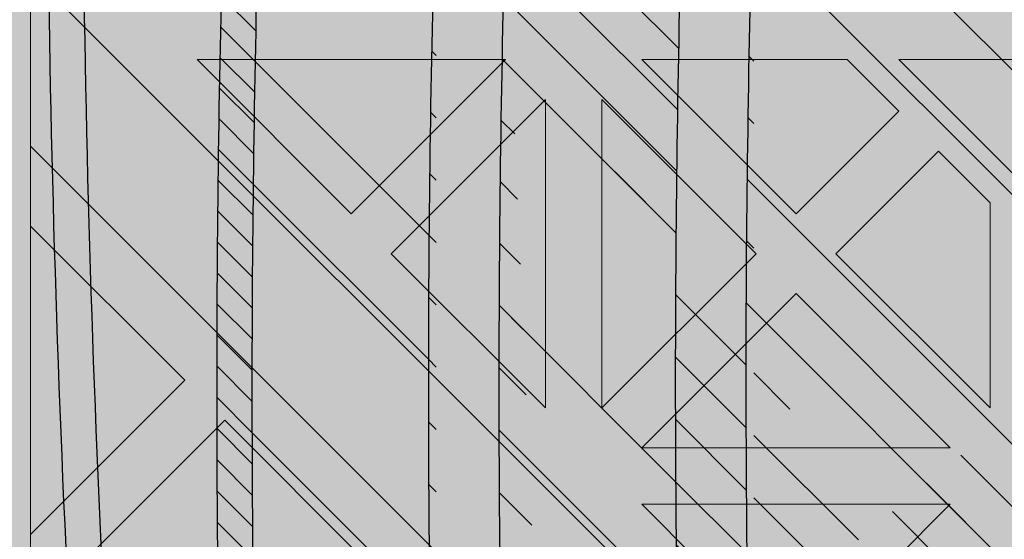
# Model space of a CAD drawing. Units: inches. Extents: x 844 to 2234, y 346 to 1084.
# Tile 28 of 93: x 1252.862 to 1257.311, y 693.415 to 695.763. Entities that reach past the tile are written whole.
import ezdxf

# ---------------------------------------------------------------- set-up
doc = ezdxf.new("R2010")
doc.units = ezdxf.units.IN
doc.header["$MEASUREMENT"] = 0
doc.layers.add('furniture', color=8, linetype='Continuous', lineweight=18)
doc.layers.add('RA-AP-01$0$INT', color=35, linetype='Continuous', lineweight=5)
doc.layers.add('RA-AP-01$0$FURN', color=3, linetype='Continuous')
doc.layers.add('RA-AP-01$0$WOOD', color=64, linetype='Continuous')

# ---------------------------------------------------------------- blocks, each defined once
blk = doc.blocks.new('A$C18D01794')
at = {"layer": 'RA-AP-01$0$INT'}
blk.add_hatch(color=256, dxfattribs=at).paths.add_polyline_path([(4.505206456958071, -6.306712009588038), (5.305206456958072, -6.306712009588038), (5.305206456958072, -7.106712009588038), (5.255206456951893, -7.10671200958804), (5.25520645694868, -6.356712009605972), (4.555206456959269, -6.356712009587461), (4.555206456956052, -7.106712009588038), (4.505206456958073, -7.106712009588038)])
h = blk.add_hatch(color=256, dxfattribs=at)
h.paths.add_polyline_path([(4.585917135068449, -6.356712009588271), (4.555206456959269, -6.35671200958746), (4.555206456959137, -6.387422687716308), (4.874495778835233, -6.706712009592356), (4.90520645695423, -6.676001331474049)])
h.paths.add_polyline_path([(5.255206456948813, -6.387422687716306), (5.255206456948682, -6.356712009605972), (5.224495778822613, -6.356712009605161), (4.905206456953498, -6.676001331474273), (4.935917135072151, -6.706712009592924)])
h.paths.add_polyline_path([(4.935917135072559, -6.706712009592068), (4.905206456953564, -6.737422687710376), (5.255206456951813, -7.087422687708613), (5.255206456951549, -7.026001331471008)])
h.paths.add_polyline_path([(4.555206456956399, -7.026001331471013), (4.555206456956134, -7.087422687708616), (4.905206456953821, -6.737422687710943), (4.874495778835166, -6.70671200959229)])
h = blk.add_hatch(color=256, dxfattribs=at)
h.paths.add_polyline_path([(4.585917135068448, -6.356712009588273), (4.614201406330596, -6.356712009589021), (4.668846067270487, -6.411356670531338), (4.723490728212344, -6.356712009591912), (4.771774999457151, -6.35671200959319), (4.826419660396886, -6.411356670535356), (4.862780050090322, -6.374996280843536), (4.844495778842715, -6.356712009595112), (4.862780050090411, -6.356712009595595), (4.905206456960182, -6.399138416468211), (4.947632863832445, -6.356712009597838), (4.965917135079675, -6.356712009598322), (4.947632863831759, -6.374996280845421), (4.983993253523576, -6.411356670538857), (5.038637914464627, -6.356712009600247), (5.08692218571208, -6.356712009601523), (5.141566846649976, -6.411356670541852), (5.196211507589851, -6.356712009604411), (5.224495778822615, -6.356712009605161), (4.905206456953975, -6.676001331473793)])
h.paths.add_polyline_path([(4.895206456956031, -6.637717060225675), (4.895206456958921, -6.528427738347902), (4.840561796018589, -6.583072399285802)], flags=16)
h.paths.add_polyline_path([(4.915206456955638, -6.637717060226121), (4.969851117895509, -6.583072399288678), (4.915206456957609, -6.528427738348344)], flags=16)
h.paths.add_polyline_path([(4.826419660395175, -6.568930263661755), (4.881064321335613, -6.514285602723745), (4.771774999456703, -6.514285602720857)], flags=16)
h.paths.add_polyline_path([(4.983993253519558, -6.568930263665262), (5.038637914460456, -6.514285602726792), (4.929348592581548, -6.514285602724816)], flags=16)
h.paths.add_polyline_path([(4.881064321336025, -6.494285602723742), (4.826419660397532, -6.439640941782821), (4.771774999457062, -6.494285602720859)], flags=16)
h.paths.add_polyline_path([(4.929348592582019, -6.494285602724817), (5.038637914460982, -6.494285602726792), (4.983993253522945, -6.439640941786327)], flags=16)
h.paths.add_polyline_path([(4.895206456960191, -6.480143467100443), (4.895206456962115, -6.407422687715913), (4.876922185715016, -6.389138416467584), (4.840561796021581, -6.425498806159401)], flags=16)
h.paths.add_polyline_path([(4.915206456958487, -6.480143467100889), (4.969851117899527, -6.425498806162279), (4.933490728206909, -6.389138416468043), (4.9152064569598, -6.40742268771434)], flags=16)
h.paths.add_polyline_path([(4.757632863832376, -6.480143467096812), (4.812277524772842, -6.425498806158772), (4.757632863834348, -6.370854145217844)], flags=16)
h.paths.add_polyline_path([(4.737632863832376, -6.480143467096286), (4.737632863834348, -6.370854145217375), (4.682988202893906, -6.425498806155385)], flags=16)
h.paths.add_polyline_path([(5.05278005008503, -6.480143467103376), (5.052780050087917, -6.370854145224413), (4.998135389146995, -6.425498806162908)], flags=16)
h.paths.add_polyline_path([(5.072780050085024, -6.480143467103744), (5.127424711025931, -6.42549880616527), (5.072780050087916, -6.370854145224832)], flags=16)
h.paths.add_polyline_path([(4.935917135072783, -6.706712009592292), (5.255206456948811, -6.387422687716309), (5.255206456948932, -6.415706958964177), (5.200561796010279, -6.470351619902839), (5.255206456949403, -6.524996280841948), (5.25520645694961, -6.5732805520894), (5.200561796009787, -6.627925213029239), (5.236922185702417, -6.664285602721864), (5.255206456949919, -6.646001331474357), (5.255206456949998, -6.664285602721898), (5.212780050078687, -6.706712009592262), (5.25520645695036, -6.749138416463932), (5.255206456950438, -6.767422687711313), (5.236922185702424, -6.749138416463297), (5.200561796009796, -6.785498806155928), (5.255206456950753, -6.840143467096874), (5.25520645695096, -6.888427738341682), (5.200561796010322, -6.943072399282328), (5.255206456951428, -6.997717060223427), (5.255206456951547, -7.026001331471006)])
h.paths.add_polyline_path([(5.042988202883395, -6.785498806155427), (5.097632863823085, -6.840143467095101), (5.097632863822622, -6.730854145216193)], flags=16)
h.paths.add_polyline_path([(5.028846067259663, -6.771356670531693), (5.083490728198774, -6.716712009592573), (4.974201406321001, -6.716712009593042)], flags=16)
h.paths.add_polyline_path([(5.117632863823087, -6.840143467095186), (5.172277524762331, -6.785498806155926), (5.11763286382262, -6.730854145216225)], flags=16)
h.paths.add_polyline_path([(5.08349072819877, -6.696712009593886), (5.028846067259652, -6.642067348654775), (4.974201406320998, -6.696712009593438)], flags=16)
h.paths.add_polyline_path([(5.131774999446817, -6.854285602718917), (5.186419660386065, -6.799640941779662), (5.241064321325782, -6.854285602719365)], flags=17)
h.paths.add_polyline_path([(5.131774999446228, -6.716712009592374), (5.186419660386065, -6.771356670532194), (5.222780050079488, -6.734996280838764), (5.204495778832781, -6.716712009592063)], flags=16)
h.paths.add_polyline_path([(5.097632863822613, -6.682569873970264), (5.097632863823061, -6.573280552091354), (5.042988202883383, -6.627925213031044)], flags=16)
h.paths.add_polyline_path([(5.131774999446899, -6.874285602718915), (5.241064321325809, -6.874285602719364), (5.186419660386591, -6.928930263658598)], flags=17)
h.paths.add_polyline_path([(5.131774999446226, -6.696712009594078), (5.204495778830767, -6.696712009594374), (5.22278005007868, -6.67842773834687), (5.186419660386049, -6.642067348654249)], flags=16)
h.paths.add_polyline_path([(5.11763286382262, -6.682569873970225), (5.17227752476232, -6.627925213030515), (5.117632863823064, -6.573280552091267)], flags=16)
h.paths.add_polyline_path([(5.186419660386069, -6.613783077405491), (5.241064321325754, -6.559138416465795), (5.131774999446791, -6.559138416466263)], flags=16)
h.paths.add_polyline_path([(5.131774999446872, -6.539138416466263), (5.24106432132578, -6.539138416465794), (5.186419660386554, -6.484493755526573)], flags=16)
h.paths.add_polyline_path([(5.255206456951811, -7.08742268770861), (5.255206456951895, -7.106712009588038), (4.555206456956052, -7.106712009588038), (4.555206456956136, -7.087422687708617), (4.905206456953973, -6.737422687710788)])
h.paths.add_polyline_path([(4.983993253513404, -6.8444937555241), (4.92934859257295, -6.899138416462108), (5.03863791445186, -6.899138416465014)], flags=16)
h.paths.add_polyline_path([(4.969851117889988, -6.83035161990006), (4.915206456952556, -6.775706958960171), (4.915206456949648, -6.884996280837944)], flags=16)
h.paths.add_polyline_path([(4.929348592572535, -6.919138416462105), (4.983993253511019, -6.973783077403037), (5.038637914451496, -6.919138416465012)], flags=16)
h.paths.add_polyline_path([(5.052780050074912, -6.93328055208906), (4.998135389134438, -6.987925213027088), (5.052780050072919, -7.042569873968025)], flags=16)
h.paths.add_polyline_path([(5.07278005007491, -6.933280552089588), (5.072780050072918, -7.042569873968497), (5.127424711013374, -6.987925213030498)], flags=16)
h.paths.add_polyline_path([(4.89520645695295, -6.775706958959721), (4.840561796013067, -6.830351619897157), (4.895206456950961, -6.884996280837494)], flags=16)
h.paths.add_polyline_path([(4.915206456948365, -6.933280552085403), (4.915206456946434, -7.006001331471951), (4.933490728192729, -7.024285602719066), (4.969851117886972, -6.987925213026453)], flags=16)
h.paths.add_polyline_path([(4.881064321327021, -6.899138416461022), (4.82641966038902, -6.84449375552057), (4.771774999448108, -6.899138416459029)], flags=16)
h.paths.add_polyline_path([(4.895206456950073, -6.933280552084951), (4.840561796009022, -6.987925213023558), (4.876922185700835, -7.024285602716997), (4.895206456948749, -7.006001331469487)], flags=16)
h.paths.add_polyline_path([(4.983993253510392, -7.0020673486505), (4.947632863816944, -7.038427738342319), (4.965917135064043, -7.05671200959023), (5.038637914448995, -7.056712009591555)], flags=16)
h.paths.add_polyline_path([(4.881064321326543, -6.91913841646102), (4.771774999447578, -6.919138416459031), (4.826419660385607, -6.973783077399508)], flags=16)
h.paths.add_polyline_path([(4.905206456946447, -7.014285602717636), (4.862780050074785, -7.056712009588352), (4.947632863816685, -7.056712009589775)], flags=16)
h.paths.add_polyline_path([(5.14156684663679, -7.002067348654549), (5.086922185696452, -7.056712009592438), (5.196211507574223, -7.056712009594425)], flags=16)
h.paths.add_polyline_path([(4.8264196603837, -7.002067348646972), (4.771774999442643, -7.056712009585575), (4.8444957788276, -7.056712009587508), (4.862780050075511, -7.038427738340416)], flags=16)
h.paths.add_polyline_path([(4.812277524760289, -6.98792521302292), (4.757632863822258, -6.933280552082447), (4.757632863819352, -7.042569873961408)], flags=16)
h.paths.add_polyline_path([(4.73763286382226, -6.933280552082079), (4.682988202881349, -6.987925213020536), (4.737632863819352, -7.04256987396099)], flags=16)
h.paths.add_polyline_path([(4.723490728195188, -7.056712009584289), (4.668846067257299, -7.002067348643949), (4.614201406317417, -7.056712009581383)], flags=16)
h.paths.add_polyline_path([(4.597632863829262, -6.706712009592262), (4.555206456957951, -6.664285602721896), (4.555206456958029, -6.646001331474357), (4.573490728205535, -6.664285602721864), (4.609851117898167, -6.627925213029238), (4.555206456958338, -6.573280552089402), (4.555206456958546, -6.524996280841952), (4.60985111789767, -6.470351619902839), (4.555206456959015, -6.415706958964177), (4.555206456959138, -6.387422687716309), (4.874495778835167, -6.70671200959229), (4.5552064569564, -7.026001331471015), (4.555206456956523, -6.997717060223433), (4.609851117897629, -6.94307239928233), (4.555206456956988, -6.888427738341681), (4.555206456957198, -6.840143467096881), (4.609851117898153, -6.78549880615593), (4.573490728205528, -6.749138416463297), (4.555206456957507, -6.76742268771132), (4.555206456957585, -6.749138416463933)])
h.paths.add_polyline_path([(4.712780050085332, -6.730854145216195), (4.712780050084863, -6.840143467095105), (4.767424711024555, -6.785498806155427)], flags=16)
h.paths.add_polyline_path([(4.726922185709173, -6.716712009592573), (4.781566846648288, -6.771356670531693), (4.836211507586949, -6.716712009593043)], flags=16)
h.paths.add_polyline_path([(4.692780050085327, -6.730854145216225), (4.638135389145619, -6.785498806155928), (4.692780050084865, -6.840143467095185)], flags=16)
h.paths.add_polyline_path([(4.726922185709182, -6.696712009593886), (4.836211507586949, -6.696712009593436), (4.7815668466483, -6.642067348654773)], flags=16)
h.paths.add_polyline_path([(4.678637914461726, -6.71671200959237), (4.605917135075169, -6.716712009592063), (4.587632863828464, -6.734996280838766), (4.623993253521887, -6.771356670532195)], flags=16)
h.paths.add_polyline_path([(4.712780050085336, -6.68256987397026), (4.767424711024568, -6.627925213031042), (4.71278005008489, -6.573280552091352)], flags=16)
h.paths.add_polyline_path([(4.678637914461726, -6.696712009594076), (4.623993253521899, -6.642067348654247), (4.587632863829271, -6.67842773834687), (4.605917135077185, -6.696712009594376)], flags=16)
h.paths.add_polyline_path([(4.692780050085336, -6.682569873970228), (4.692780050084889, -6.573280552091267), (4.638135389145632, -6.627925213030515)], flags=16)
h.paths.add_polyline_path([(4.623993253521885, -6.799640941779662), (4.678637914461131, -6.854285602718915), (4.56934859258217, -6.854285602719365)], flags=17)
h.paths.add_polyline_path([(4.623993253521901, -6.613783077405509), (4.678637914461158, -6.559138416466263), (4.569348592582195, -6.559138416465795)], flags=16)
h.paths.add_polyline_path([(4.678637914461051, -6.874285602718915), (4.623993253521361, -6.928930263658598), (4.569348592582143, -6.874285602719364)], flags=17)
h.paths.add_polyline_path([(4.678637914461076, -6.539138416466263), (4.623993253521399, -6.484493755526573), (4.569348592582167, -6.539138416465796)], flags=16)
h = blk.add_hatch(color=256, dxfattribs=at)
h.paths.add_polyline_path([(5.028846067259997, -6.642067348655121), (4.974201406321342, -6.696712009593783), (5.083490728199115, -6.69671200959423)])
h.paths.add_polyline_path([(4.974201406321344, -6.716712009593388), (5.028846067260004, -6.771356670532039), (5.083490728199117, -6.716712009592919)])
h.paths.add_polyline_path([(5.042988202883738, -6.785498806155768), (5.097632863823428, -6.840143467095449), (5.097632863822963, -6.73085414521654)])
h.paths.add_polyline_path([(5.117632863822961, -6.730854145216568), (5.117632863823428, -6.840143467095531), (5.172277524762674, -6.785498806156272)])
h.paths.add_polyline_path([(5.131774999446572, -6.716712009592718), (5.186419660386406, -6.77135667053254), (5.222780050079831, -6.734996280839116), (5.204495778833122, -6.716712009592409)])
h.paths.add_polyline_path([(5.236922185702764, -6.749138416463644), (5.200561796010139, -6.785498806156274), (5.255206456949971, -6.840143467096101), (5.255206456950271, -6.76742268771115)])
h.paths.add_polyline_path([(5.186419660386412, -6.799640941780006), (5.131774999447164, -6.854285602719262), (5.241064321326123, -6.854285602719711)])
h.paths.add_polyline_path([(5.131774999447238, -6.874285602719261), (5.186419660386934, -6.928930263658944), (5.241064321326153, -6.874285602719709)])
h.paths.add_polyline_path([(5.200561796010663, -6.943072399282675), (5.255206456949324, -6.997717060221329), (5.255206456949777, -6.888427738343558)])
h.paths.add_polyline_path([(5.21278005007903, -6.706712009592607), (5.255206456950223, -6.749138416463798), (5.255206456950696, -6.664285602721891)])
h.paths.add_polyline_path([(5.13177499944657, -6.696712009594424), (5.204495778831106, -6.696712009594723), (5.222780050079024, -6.678427738347219), (5.186419660386397, -6.642067348654592)])
h.paths.add_polyline_path([(5.117632863823405, -6.573280552091611), (5.117632863822955, -6.682569873970578), (5.172277524762665, -6.627925213030859)])
h.paths.add_polyline_path([(5.042988202883727, -6.627925213031387), (5.097632863822957, -6.682569873970603), (5.097632863823407, -6.573280552091697)])
h.paths.add_polyline_path([(5.131774999447135, -6.559138416466609), (5.186419660386394, -6.613783077405857), (5.241064321326097, -6.559138416466144)])
h.paths.add_polyline_path([(5.200561796010128, -6.627925213029584), (5.236922185702758, -6.664285602722211), (5.255206456950264, -6.646001331474705), (5.255206456949948, -6.573280552089752)])
h.paths.add_polyline_path([(5.186419660386895, -6.484493755526919), (5.131774999447213, -6.539138416466609), (5.241064321326127, -6.539138416466142)])
h.paths.add_polyline_path([(5.200561796010624, -6.470351619903183), (5.255206456949745, -6.524996280842298), (5.255206456949276, -6.415706958964523)])
h = blk.add_hatch(color=256, dxfattribs=at)
h.paths.add_polyline_path([(4.895206456952951, -6.77570695895972), (4.840561796013068, -6.830351619897156), (4.895206456950958, -6.884996280837495)])
h.paths.add_polyline_path([(4.915206456949649, -6.884996280837942), (4.969851117889987, -6.830351619900054), (4.915206456952556, -6.775706958960171)])
h.paths.add_polyline_path([(5.038637914451862, -6.899138416465013), (4.983993253513403, -6.8444937555241), (4.929348592572953, -6.899138416462106)])
h.paths.add_polyline_path([(4.929348592572535, -6.919138416462105), (4.983993253511018, -6.973783077403037), (5.038637914451497, -6.919138416465012)])
h.paths.add_polyline_path([(4.915206456948366, -6.933280552085397), (4.915206456946433, -7.006001331471951), (4.93349072819273, -7.024285602719068), (4.969851117886972, -6.987925213026454)])
h.paths.add_polyline_path([(5.038637914448995, -7.056712009591553), (4.983993253510389, -7.002067348650502), (4.947632863816946, -7.038427738342318), (4.965917135064043, -7.05671200959023)])
h.paths.add_polyline_path([(5.05278005007292, -7.042569873968023), (5.05278005007491, -6.933280552089059), (4.998135389134438, -6.987925213027088)])
h.paths.add_polyline_path([(5.07278005007292, -7.042569873968496), (5.127424711013374, -6.987925213030498), (5.072780050074909, -6.933280552089588)])
h.paths.add_polyline_path([(5.141566846636789, -7.002067348654547), (5.086922185696449, -7.056712009592438), (5.196211507574223, -7.056712009594425)])
h.paths.add_polyline_path([(4.947632863816688, -7.056712009589774), (4.905206456946449, -7.014285602717634), (4.862780050074784, -7.056712009588353)])
h.paths.add_polyline_path([(4.840561796009025, -6.987925213023556), (4.876922185700834, -7.024285602716997), (4.895206456948747, -7.006001331469488), (4.895206456950075, -6.933280552084953)])
h.paths.add_polyline_path([(4.88106432132654, -6.919138416461021), (4.771774999447577, -6.919138416459031), (4.826419660385606, -6.973783077399508)])
h.paths.add_polyline_path([(4.881064321327019, -6.899138416461022), (4.826419660389019, -6.844493755520571), (4.771774999448108, -6.89913841645903)])
h.paths.add_polyline_path([(4.757632863819352, -7.042569873961409), (4.812277524760284, -6.987925213022922), (4.757632863822259, -6.933280552082447)])
h.paths.add_polyline_path([(4.8264196603837, -7.002067348646974), (4.771774999442646, -7.056712009585575), (4.844495778827599, -7.05671200958751), (4.862780050075512, -7.038427738340417)])
h.paths.add_polyline_path([(4.737632863819352, -7.042569873960988), (4.737632863822258, -6.933280552082078), (4.682988202881349, -6.987925213020538)])
h.paths.add_polyline_path([(4.668846067257299, -7.002067348643952), (4.61420140631742, -7.056712009581384), (4.723490728195189, -7.056712009584292)])
for p, q in [((5.255206456951895, -7.106712009588038), (5.255206456948681, -6.356712009605972)), ((4.935917135072783, -6.706712009592292), (5.255206456951548, -7.026001331471007)), ((4.905206456953975, -6.737422687710788), (5.255206456951811, -7.087422687708611)), ((4.929348592572952, -6.899138416462106), (4.983993253513403, -6.844493755524101)), ((4.983993253513404, -6.844493755524103), (5.038637914451862, -6.899138416465012)), ((5.186419660386587, -6.928930263658596), (5.131774999446899, -6.874285602718915)), ((5.241064321325809, -6.874285602719364), (5.186419660386589, -6.928930263658598)), ((5.255206456949429, -6.888427738343214), (5.200561796010322, -6.943072399282328)), ((5.255206456949433, -6.888427738343212), (5.255206456948982, -6.997717060220983)), ((5.038637914451862, -6.899138416465012), (4.929348592572952, -6.899138416462106)), ((5.038637914451498, -6.919138416465012), (4.929348592572535, -6.919138416462105)), ((4.929348592572535, -6.919138416462105), (4.983993253511019, -6.973783077403037)), ((5.038637914451498, -6.919138416465012), (4.983993253511019, -6.973783077403037)), ((4.915206456946434, -7.006001331470351), (4.915206456948367, -6.933280552085399)), ((4.915206456948367, -6.933280552085399), (4.969851117886972, -6.987925213026453)), ((5.05278005007491, -6.93328055208906), (4.998135389134438, -6.987925213027088)), ((5.05278005007491, -6.93328055208906), (5.052780050072921, -7.042569873968023)), ((5.127424711013373, -6.987925213030496), (5.07278005007491, -6.933280552089588)), ((5.07278005007491, -6.933280552089588), (5.07278005007292, -7.042569873968497)), ((5.255206456948982, -6.997717060220983), (5.200561796010322, -6.943072399282328)), ((4.969851117886972, -6.987925213026452), (4.93349072819353, -7.024285602718265)), ((5.052780050072921, -7.042569873968023), (4.998135389134438, -6.987925213027088)), ((5.07278005007292, -7.042569873968497), (5.127424711013374, -6.987925213030498)), ((4.98399325351039, -7.002067348650502), (4.947632863816946, -7.038427738342317)), ((5.038637914448995, -7.056712009591555), (4.983993253510388, -7.002067348650502)), ((5.086922185696454, -7.056712009592434), (5.141566846636789, -7.002067348654547)), ((5.196211507574223, -7.056712009594425), (5.141566846636789, -7.002067348654547)), ((4.915206456946427, -7.006001331471944), (4.933490728193524, -7.02428560271986)), ((4.905206456946449, -7.014285602717635), (4.94763286381669, -7.056712009589775)), ((4.947632863816946, -7.038427738342317), (4.965917135063997, -7.056712009590183)), ((4.965917135064043, -7.056712009590231), (4.947632863816944, -7.038427738342317)), ((4.94763286381669, -7.056712009589775), (4.862780050074783, -7.056712009588354)), ((4.965917135064043, -7.05671200959023), (5.038637914448995, -7.056712009591555)), ((5.086922185696452, -7.056712009592438), (5.196211507574223, -7.056712009594425))]:
    blk.add_line(p, q, dxfattribs=at)
blk = doc.blocks.new('A$C32926AE1')
at = {"layer": 'RA-AP-01$0$FURN'}
h = blk.add_hatch(dxfattribs=at)
h.set_pattern_fill('ANSI31', color=256, scale=0.1, style=0)
h.set_pattern_definition([(45, (0, 0), (-0.0088388347648318, 0.0088388347648318), [])])
edge = h.paths.add_edge_path(flags=16)
edge.add_arc((4.904771284329206, 4.246793130718756), 0.2603971832811541, 75.22398030683196, 104.7760196931204)
edge.add_arc((4.904771284329206, 4.246793130718756), 0.2603971832811541, 75.223980306832, 104.77601969312039, ccw=False)
edge = h.paths.add_edge_path(flags=16)
edge.add_arc((4.904771284329206, 4.067062675376612), 0.2603971832811541, 255.2239803068796, 284.776019693168)
edge.add_arc((4.904771284329206, 4.067062675376612), 0.2603971832811541, 255.22398030687958, 284.77601969316805, ccw=False)
edge = h.paths.add_edge_path(flags=0)
edge.add_arc((4.904771284329206, 4.067062675376612), 0.2603971832811541, 255.2239803068796, 284.776019693168)
edge.add_arc((4.904771284329206, 4.067062675376612), 0.2603971832811541, 255.22398030687958, 284.77601969316805, ccw=False)
edge = h.paths.add_edge_path(flags=0)
edge.add_arc((4.904771284329206, 4.067062675376612), 0.2603971832811541, 255.2239803068796, 284.776019693168)
edge.add_arc((4.904771284329206, 4.067062675376612), 0.2603971832811541, 255.22398030687958, 284.77601969316805, ccw=False)
edge = h.paths.add_edge_path()
edge.add_arc((4.604388392048174, 4.588829985554312), 0.1599999999999918, 342.3781640246255, 354.4317409793762)
edge.add_arc((5.090145208887507, 4.43216705527679), 0.3503971832811637, 162.0091218307731, 180.3186872093483)
edge.add_arc((5.205154176610243, 4.588829985554953), 0.1599999999999917, 185.5682590208461, 197.6218359767349)
edge.add_arc((4.904771284329229, 4.246793130718735), 0.3503971832811761, 72.00912183053516, 107.9908781690354)
edge.add_arc((9.535952835716557, 4.28682295566602), 4.798342501046485, 178.2875002453811, 181.5576802719453)
edge.add_arc((4.719397359771122, 4.43216705527679), 0.3503971832811637, 359.6813127906516, 377.9908781692269)
edge.add_arc((9.535967292294904, 4.286822350292874), 4.778371420254705, 178.2965938931842, 181.5667745797229)
edge.add_arc((4.719397359771122, 4.43216705527679), 0.3303971832811637, 359.6813127906516, 377.9908781692269)
edge.add_arc((0.2735752763637294, 4.286822350292874), 4.7783714202547, 358.4332254202771, 361.7034061068158)
edge.add_arc((5.061434214606998, 4.732549947558029), 0.1600000000000254, 252.3781640250584, 264.4317409792362)
edge.add_arc((4.748108354051257, 4.732549947558012), 0.1600000000000541, 275.5682590208426, 287.6218359759532)
edge.add_arc((4.604388392048115, 4.588829985554317), 0.1800000000000505, 342.3567572500182, 349.3735009646207)
edge.add_arc((5.205154176610254, 4.588829985554976), 0.1800000000000069, 190.6264990356027, 197.6432427513933)
edge.add_arc((5.061434214607106, 4.732549947558013), 0.1800000000000424, 252.3567572496606, 259.3735009644582)
edge.add_arc((4.904771284329208, 4.246793130718737), 0.3303971832811676, 71.99844483668534, 108.0015551637021)
edge.add_arc((4.748108354051414, 4.732549947558045), 0.1800000000000547, 280.6264990355479, 287.6432427495938)
edge.add_arc((5.090145208887514, 4.432167055276789), 0.2803971832811691, 162.8706300666893, 180.816523289902)
edge.add_arc((4.719397359771136, 4.432167055276689), 0.2803971832811534, 359.183476710103, 377.1293699333214)
edge.add_arc((4.904771284329222, 4.246793130718737), 0.2803971832811769, 72.87063006672916, 107.1293699332334)
edge.add_arc((5.090145208887522, 4.432167055276788), 0.2603971832811776, 165.2239803068007, 180.9953123810312)
edge.add_arc((4.719397359771141, 4.432167055276699), 0.2603971832811458, 359.0046876189768, 374.7760196932087)
edge.add_arc((5.090145208887507, 4.43216705527679), 0.3303971832811637, 162.0091218307731, 180.3186872093483)
edge.add_arc((9.53595427642584, 4.285015535491528), 4.728345371032053, 178.265043920078, 181.5679956281801)
edge.add_arc((0.2735882922327999, 4.285015535491582), 4.728345371032045, 358.4320043718193, 361.7349560799204)
edge.add_arc((9.535953591267507, 4.284458026472751), 4.708343996644348, 178.2573054306777, 181.5704995759608)
edge.add_arc((0.273588977391114, 4.284458026472785), 4.708343996644358, 358.4295004240388, 361.7426945693213)
edge.add_arc((0.2735889773911131, 4.029397779622582), 4.708343996644359, 358.2573054306787, 361.5704995759613)
edge.add_arc((9.535953591267518, 4.029397779622618), 4.708343996644359, 178.4295004240391, 181.7426945693223)
edge.add_arc((0.2735882922327901, 4.028840270603786), 4.728345371032054, 358.2650439200796, 361.5679956281808)
edge.add_arc((9.53595427642584, 4.028840270603841), 4.728345371032054, 178.4320043718199, 181.7349560799219)
edge.add_arc((0.2735752763637302, 4.027033455802493), 4.778371420254699, 358.2965938931842, 361.5667745797229)
edge.add_arc((4.719397359771122, 3.881688750818578), 0.3303971832811637, 342.0091218307731, 360.3186872093484)
edge.add_arc((5.090145208887507, 3.881688750818578), 0.3303971832811637, 179.6813127906516, 197.9908781692269)
edge.add_arc((9.535967292294904, 4.027033455802493), 4.778371420254705, 178.433225420277, 181.7034061068158)
edge.add_arc((4.719397359771122, 3.881688750818578), 0.3503971832811637, 342.0091218307731, 360.3186872093484)
edge.add_arc((9.53595283571655, 4.027032850429349), 4.79834250104648, 178.4423197280546, 181.7124997546188)
edge.add_arc((4.719397359771141, 3.881688750818669), 0.2603971832811458, 345.2239803067913, 360.9953123810232)
edge.add_arc((5.090145208887522, 3.88168875081858), 0.2603971832811776, 179.0046876189687, 194.7760196931993)
edge.add_arc((4.904771284329222, 4.067062675376631), 0.2803971832811769, 252.8706300667665, 287.1293699332708)
edge.add_arc((4.719397359771136, 3.881688750818678), 0.2803971832811534, 342.8706300666787, 360.8165232898969)
edge.add_arc((5.090145208887514, 3.881688750818579), 0.2803971832811691, 179.183476710098, 197.1293699333106)
edge.add_arc((4.748108354051414, 3.581305858537323), 0.1800000000000547, 72.3567572504062, 79.37350096445199)
edge.add_arc((4.904771284329208, 4.067062675376631), 0.3303971832811676, 251.9984448362979, 288.0015551633146)
edge.add_arc((5.061434214607106, 3.581305858537355), 0.1800000000000424, 100.6264990355418, 107.6432427503394)
edge.add_arc((5.205154176610254, 3.725025820540392), 0.1800000000000069, 162.3567572486066, 169.3735009643972)
edge.add_arc((4.604388392048115, 3.725025820541051), 0.1800000000000505, 10.62649903537925, 17.64324274998182)
edge.add_arc((4.748108354051257, 3.581305858537356), 0.1600000000000541, 72.37816402404681, 84.43174097915735)
edge.add_arc((4.904771284329229, 4.067062675376632), 0.3503971832811761, 252.0091218309645, 287.9908781694648)
edge.add_arc((5.061434214606998, 3.581305858537339), 0.1600000000000254, 95.56825902076373, 107.6218359749416)
edge.add_arc((5.205154176610243, 3.725025820540414), 0.1599999999999917, 162.3781640232651, 174.4317409791539)
edge.add_arc((5.090145208887507, 3.881688750818578), 0.3503971832811637, 179.6813127906516, 197.9908781692269)
edge.add_arc((4.604388392048174, 3.725025820541056), 0.1599999999999918, 5.568259020623824, 17.62183597537444)
edge.add_arc((0.2735897329420762, 4.28682295566602), 4.798342501046482, 358.4423197280547, 361.7124997546188)
edge.add_arc((0.2735897329420691, 4.027032850429348), 4.798342501046489, 358.2875002453812, 361.5576802719453)
at = {"layer": 'RA-AP-01$0$WOOD'}
h = blk.add_hatch(color=256, dxfattribs=at)
h.dxf.hatch_style = 1
h.paths.add_polyline_path([(5.157430609644524, 4.573483066760929, -0.1009492694046607), (5.155401577623758, 4.593365984175333, -0.1842662638101597), (5.172249623284174, 4.638795604568598, 0.2056608120311276), (5.179560981299304, 4.661316324430096, 0.3614336704623542), (5.134352340494423, 4.706524965234944, 0.2056608120311297), (5.111831620632933, 4.699213607219793, -0.1842662638101113), (5.066402000239693, 4.682365561559342, -0.1055311479399994), (5.045656153913092, 4.68467289944697, 0.1567636581983829), (4.763886414745334, 4.684672899446966, -0.1055311479399895), (4.743140568418733, 4.68236556155934, -0.1842662638100833), (4.6977109480255, 4.69921360721979, 0.2056608120302612), (4.675190228164109, 4.706524965234949, 0.3614336704708441), (4.629981587358889, 4.66131632442871, 0.2056608120245944), (4.637292945374126, 4.638795604567974, -0.1842662638101024), (4.654140991034615, 4.59336598417475, -0.1009492694055169), (4.652111959013835, 4.573483066760181, 0.021410119221476), (4.629748025606143, 4.156712009541676, 0.0214101192214795), (4.652111959013809, 3.739940952323101, -0.1009492694059586), (4.654140991034615, 3.720058034908448, -0.1842662638100975), (4.637292945374126, 3.674628414515226, 0.2056608120245705), (4.629981587358889, 3.652107694654492, 0.3614336704708879), (4.675190228164113, 3.606899053848249, 0.2056608120302384), (4.697710948025501, 3.614210411863408, -0.1842662638100995), (4.743140568418738, 3.63105845752386, -0.1055311479402541), (4.763886414745388, 3.628751119636215, 0.1567636581983776), (5.045656153913137, 3.628751119636244, -0.1055311479397538), (5.066402000239692, 3.631058457523857, -0.1842662638101067), (5.111831620632931, 3.614210411863407, 0.2056608120310924), (5.134352340494417, 3.606899053848256, 0.3614336704624001), (5.179560981299307, 3.652107694653103, 0.2056608120311314), (5.172249623284175, 3.6746284145146, -0.1842662638101402), (5.155401577623758, 3.72005803490786, -0.1009492694051366), (5.15743060964455, 3.739940952322354, 0.0214101192215073), (5.179794543052287, 4.156712009541468, 0.0214101192215252)])
h.paths.add_polyline_path([(4.639748609479751, 4.156712009541513, 0.0213537860821624), (4.661970494867118, 3.741887061152232, -0.094075836301374), (4.664143710413708, 3.7196126951003, -0.1824818158568985), (4.644813765429836, 3.668037719127816, 0.2056608120245319), (4.639939526753007, 3.653023905887301, 0.3614336704710246), (4.676106439397173, 3.616856993242342, 0.2056608120302234), (4.691120252638095, 3.621731231919122, -0.1824818158602558), (4.742695228611606, 3.641061176902986, -0.1029891339458722), (4.766991894714349, 3.638256818950944, 0.156709409989566), (5.042550673941472, 3.638256818950105, -0.102989133958497), (5.066847340047078, 3.641061176902949, -0.1824818158594995), (5.118422316020358, 3.621731231919103, 0.2056608120311416), (5.133436129261316, 3.616856993242346, 0.3614336704621468), (5.169603041905217, 3.653023905886178, 0.2056608120310986), (5.164728803228477, 3.668037719127177, -0.1824818158565612), (5.145398858244737, 3.719612695099578, -0.0940758363009313), (5.147572073791232, 3.741887061151398, 0.0213537860822023), (5.169793959178681, 4.156712009541451, 0.0213537860822226), (5.147572073791203, 4.571536957931898, -0.0940758363005034), (5.145398858244737, 4.59381132398362, -0.1824818158565587), (5.164728803228476, 4.645386299956021, 0.2056608120311045), (5.169603041905216, 4.66040011319702, 0.3614336704621845), (5.133436129261313, 4.696567025840856, 0.2056608120310773), (5.118422316020359, 4.691692787164098, -0.182481815859508), (5.066847340047078, 4.67236284218025, -0.1029891339584606), (5.04255067394148, 4.675167200133092, 0.156709409989566), (4.766991894714357, 4.675167200132257, -0.1029891339458842), (4.742695228611611, 4.672362842180213, -0.1824818158602725), (4.691120252638095, 4.691692787164077, 0.2056608120302152), (4.676106439397174, 4.696567025840858, 0.3614336704710363), (4.639939526753005, 4.660400113195899, 0.2056608120245495), (4.644813765429837, 4.645386299955384, -0.1824818158568934), (4.664143710413708, 4.593811323982902, -0.0940758363009187), (4.661970494867149, 4.571536957931074, 0.021353786082177)], flags=16)
h.paths.add_polyline_path([(5.129794543052235, 4.432167055276933, -0.0141661062790638), (5.130152669293814, 4.156927903047693, -0.0141661062790647), (5.129794543052234, 3.881688750818433, -0.0785247771143638), (5.10979738006795, 3.755143611847103, 0.0945969212073497), (5.105408519571111, 3.717898134952927, 0.1043170707844957), (5.116074640131521, 3.670385395016088, 0.1043170707864965), (5.068561900193738, 3.681051515576561, 0.09459692119553), (5.031316423304057, 3.676662655080835, -0.1580239521427272), (4.778226145355827, 3.676662655080367, 0.0945969211986668), (4.740980668464973, 3.681051515576592, 0.1043170707882822), (4.693467928526415, 3.670385395015844, 0.1043170707867916), (4.704134049087309, 3.717898134953662, 0.0945969211972894), (4.69974518859162, 3.755143611844042, -0.0785247771163196), (4.679748025606343, 3.881688750818406, -0.0141661062790663), (4.679389899364763, 4.156927903047693, -0.0141661062790672), (4.679748025606343, 4.432167055276998, -0.0785247771163064), (4.699745188591625, 4.55871219425134, 0.094596921197333), (4.704134049087308, 4.595957671141738, 0.1043170707867205), (4.693467928526416, 4.643470411079523, 0.1043170707882628), (4.740980668464965, 4.632804290518776, 0.0945969211988114), (4.778226145355874, 4.637193151015016, -0.158023952142669), (5.031316423304015, 4.637193151014546, 0.0945969211956361), (5.068561900193736, 4.632804290518806, 0.1043170707864979), (5.11607464013152, 4.643470411079278, 0.1043170707844617), (5.105408519571112, 4.595957671142455, 0.0945969212074597), (5.109797380067959, 4.558712194248236, -0.0785247771143467)], flags=0)
h.paths.add_polyline_path([(5.119794532311105, 4.432259799204851, -0.0142000800617244), (5.120156169157484, 4.156927903047701, -0.0142000800617277), (5.119794532311105, 3.881596006890482, -0.0784894509520253), (5.100273383573699, 3.758192358677797, 0.0940138827242913), (5.095413455884425, 3.717477693979438, 0.0606271852308753), (5.099615656341024, 3.686844378806616, 0.0606271852322524), (5.068982341167493, 3.691046579263239, 0.0940138827010453), (5.028267676478798, 3.686186651576848, -0.1580706864508061), (4.781274892180912, 3.686186651576435, 0.0940138827026903), (4.740560227491556, 3.691046579263279, 0.0606271852339895), (4.709926912317155, 3.686844378806508, 0.0606271852329405), (4.714129112773991, 3.717477693980356, 0.094013882701304), (4.709269185087677, 3.758192358669163, -0.0784894509577193), (4.689748036347473, 3.881596006890469, -0.014200080061729), (4.689386399501094, 4.156927903047709, -0.0142000800617217), (4.689748036347473, 4.432259799204808, -0.078489450957724), (4.709269185087651, 4.555663447426125, 0.0940138827014585), (4.714129112773992, 4.596378112114996, 0.0606271852329731), (4.709926912317154, 4.62701142728886, 0.0606271852340196), (4.74056022749157, 4.622809226832087, 0.0940138827024997), (4.781274892180847, 4.627669154518912, -0.1580706864508359), (5.028267676478777, 4.627669154518526, 0.0940138827010946), (5.068982341167492, 4.622809226832129, 0.060627185232254), (5.099615656341024, 4.627011427288751, 0.0606271852308727), (5.095413455884425, 4.59637811211593, 0.0940138827241088), (5.100273383573675, 4.555663447417647, -0.0784894509520978)], flags=0)
h.paths.add_polyline_path([(5.06978912287499, 4.430218106756144, -0.014241683694547), (5.070173729147532, 4.156927903047672, -0.0142416836945458), (5.06978912287499, 3.883637699339223, -0.0800609523125196), (5.052662118612511, 3.773463122773442, 0.0526421978001116), (5.04590916754064, 3.740550867606997, 0.0526421977992423), (5.012996912374707, 3.73379791653534, -0.1583028414718258), (4.796545656286308, 3.73379791653451, 0.0526421978034211), (4.763633401117837, 3.740550867607021, 0.0526421978018622), (4.756880450045755, 3.773463122774558, -0.0800609523117106), (4.739753445783639, 3.883637699339268, -0.0142416836945435), (4.739368839511098, 4.156927903047671, -0.0142416836945477), (4.739753445783639, 4.430218106756155, -0.0800609523116345), (4.75688045004574, 4.540392683320762, 0.052642197801941), (4.763633401117837, 4.573304938488346, 0.0526421978035071), (4.796545656286361, 4.580057889560873, -0.1583028414717561), (5.012996912374669, 4.580057889560039, 0.0526421977993048), (5.04590916754064, 4.57330493848837, 0.0526421978002057), (5.052662118612529, 4.540392683321868, -0.080060952312477)], flags=0)
h.paths.add_polyline_path([(5.049789715110557, 4.43038092723357, -0.0143097550741839), (5.05018085590259, 4.156927903047715, -0.0143097550741854), (5.049789715110558, 3.883474878861827, -0.0800685599149176), (5.03362098255317, 3.779581877367999, 0.0306258898956367), (5.028241146483733, 3.758218888663947, 0.0306258898977031), (5.006878157778253, 3.75283905259408, -0.1583983521624096), (4.802664410878162, 3.752839052594731, 0.0306258898946014), (4.781301422174808, 3.758218888663924, 0.0306258898967912), (4.775921586105202, 3.779581877368794, -0.080068559914251), (4.759752853548071, 3.883474878861786, -0.0143097550741854), (4.759361712756037, 4.156927903047671, -0.0143097550741854), (4.759752853548071, 4.430380927233557, -0.0800685599142479), (4.775921586105193, 4.534273928726546, 0.0306258898968306), (4.781301422174808, 4.555636917431444, 0.0306258898945754), (4.802664410878143, 4.561016753500631, -0.1583983521624168), (5.006878157778244, 4.561016753501291, 0.0306258898977177), (5.028241146483733, 4.555636917431421, 0.0306258898958182), (5.03362098255321, 4.534273928727244, -0.080068559914796)], flags=0)
h.paths.add_polyline_path([(4.999766070382627, 4.428171244713864, -0.0143443147609634), (5.000198441819402, 4.156927903047689, -0.0143443147609612), (4.999766070382627, 3.885684561381556, -0.0784641635803329), (4.987356730658798, 3.799103304488872, -0.1506053783831347), (4.822185837999821, 3.79910330448882, -0.0784641635803318), (4.809776498276007, 3.885684561381509, -0.014344314760963), (4.809344126839227, 4.156927903047677, -0.0143443147609645), (4.809776498276007, 4.428171244713873, -0.0784641635803192), (4.822185837999822, 4.514752501606549, -0.1506053783831338), (4.987356730658798, 4.514752501606494, -0.078464163580285)], flags=0)
h.paths.add_polyline_path([(4.979755254238824, 4.42764379880488, -0.0143772539198268), (4.980205517789977, 4.156927903047693, -0.0143772539198275), (4.979755254238824, 3.886212007290489, -0.0689242507424422), (4.971183264704897, 3.815276770442801, -0.1296645318904179), (4.838359303953726, 3.815276770442746, -0.0689242507424186), (4.829787314419809, 3.886212007290419, -0.0143772539198292), (4.829337050868653, 4.156927903047653, -0.0143772539198325), (4.829787314419809, 4.427643798804946, -0.0689242507424211), (4.838359303953725, 4.498579035652621, -0.1296645318904187), (4.971183264704897, 4.498579035652565, -0.0689242507424401)], flags=0)
h = blk.add_hatch(color=256, dxfattribs=at)
h.dxf.hatch_style = 1
h.paths.add_polyline_path([(5.145398858244737, 4.59381132398362, -0.1824818158565616), (5.164728803228476, 4.645386299956021, 0.2056608120311045), (5.169603041905216, 4.66040011319702, 0.3614336704621845), (5.133436129261313, 4.696567025840856, 0.2056608120310773), (5.118422316020359, 4.691692787164098, -0.182481815859508), (5.066847340047078, 4.67236284218025, -0.1029891339584606), (5.04255067394148, 4.675167200133092, 0.156709409989566), (4.766991894714357, 4.675167200132257, -0.1029891339458842), (4.742695228611611, 4.672362842180213, -0.1824818158602725), (4.691120252638095, 4.691692787164077, 0.2056608120302152), (4.676106439397174, 4.696567025840858, 0.3614336704710363), (4.639939526753005, 4.660400113195899, 0.2056608120245495), (4.644813765429837, 4.645386299955384, -0.1824818158568934), (4.664143710413708, 4.593811323982902, -0.0940758363009187), (4.661970494867149, 4.571536957931074, 0.0213537860821772), (4.639748609479751, 4.156712009541507, 0.0213537860821625), (4.661970494867119, 3.741887061152226, -0.0940758363013071), (4.664143710413708, 3.719612695100309, -0.1824818158569294), (4.644813765429836, 3.668037719127816, 0.2056608120245319), (4.639939526753007, 3.653023905887301, 0.3614336704710246), (4.676106439397173, 3.616856993242342, 0.2056608120302234), (4.691120252638095, 3.621731231919122, -0.1824818158602558), (4.742695228611606, 3.641061176902986, -0.1029891339458722), (4.766991894714349, 3.638256818950944, 0.156709409989566), (5.042550673941472, 3.638256818950105, -0.102989133958497), (5.066847340047078, 3.641061176902949, -0.1824818158594995), (5.118422316020358, 3.621731231919103, 0.2056608120311416), (5.133436129261316, 3.616856993242346, 0.3614336704621468), (5.169603041905217, 3.653023905886178, 0.2056608120310986), (5.164728803228477, 3.668037719127177, -0.1824818158565612), (5.145398858244737, 3.719612695099578, -0.0940758363009313), (5.147572073791232, 3.741887061151398, 0.0213537860822023), (5.169793959178681, 4.156712009541451, 0.0213537860822226), (5.147572073791203, 4.571536957931898, -0.0940758363004996)])
h.paths.add_polyline_path([(5.109797380067958, 4.55871219424824, -0.0785247771143472), (5.129794543052234, 4.432167055276936, -0.0141661062790644), (5.130152669293814, 4.156927903047685, -0.014166106279066), (5.129794543052234, 3.881688750818401, -0.0785247771143517), (5.109797380067946, 3.755143611847092, 0.0945969212073132), (5.105408519571111, 3.717898134952929, 0.1043170707844995), (5.116074640131521, 3.670385395016088, 0.1043170707864965), (5.068561900193738, 3.681051515576561, 0.09459692119553), (5.031316423304057, 3.676662655080835, -0.1580239521427272), (4.778226145355827, 3.676662655080367, 0.0945969211986668), (4.740980668464973, 3.681051515576592, 0.1043170707882822), (4.693467928526415, 3.670385395015844, 0.1043170707867916), (4.704134049087309, 3.717898134953662, 0.0945969211972894), (4.69974518859162, 3.755143611844042, -0.0785247771163196), (4.679748025606343, 3.881688750818406, -0.0141661062790663), (4.679389899364763, 4.156927903047693, -0.0141661062790672), (4.679748025606343, 4.432167055276998, -0.0785247771163064), (4.699745188591625, 4.55871219425134, 0.094596921197333), (4.704134049087308, 4.595957671141738, 0.1043170707867205), (4.693467928526416, 4.643470411079523, 0.1043170707882628), (4.740980668464965, 4.632804290518776, 0.0945969211988114), (4.778226145355874, 4.637193151015016, -0.158023952142669), (5.031316423304015, 4.637193151014546, 0.0945969211956361), (5.068561900193736, 4.632804290518806, 0.1043170707864979), (5.11607464013152, 4.643470411079278, 0.1043170707844617), (5.105408519571112, 4.595957671142455, 0.0945969212074504)], flags=16)
h.paths.add_polyline_path([(5.100273383573655, 4.55566344741771, -0.0784894509521388), (5.119794532311105, 4.432259799204852, -0.0142000800617252), (5.120156169157484, 4.156927903047686, -0.014200080061726), (5.119794532311105, 3.881596006890502, -0.0784894509520446), (5.100273383573696, 3.758192358677786, 0.0940138827242721), (5.095413455884425, 3.717477693979436, 0.0606271852308692), (5.099615656341024, 3.686844378806616, 0.0606271852322522), (5.068982341167493, 3.691046579263239, 0.0940138827010453), (5.028267676478798, 3.686186651576848, -0.1580706864508061), (4.781274892180912, 3.686186651576435, 0.0940138827026903), (4.740560227491556, 3.691046579263279, 0.0606271852339895), (4.709926912317155, 3.686844378806508, 0.0606271852329405), (4.714129112773991, 3.717477693980356, 0.094013882701304), (4.709269185087677, 3.758192358669163, -0.0784894509577193), (4.689748036347473, 3.881596006890469, -0.014200080061729), (4.689386399501094, 4.156927903047709, -0.0142000800617217), (4.689748036347473, 4.432259799204808, -0.078489450957724), (4.709269185087651, 4.555663447426125, 0.0940138827014585), (4.714129112773992, 4.596378112114996, 0.0606271852329731), (4.709926912317154, 4.62701142728886, 0.0606271852340196), (4.74056022749157, 4.622809226832087, 0.0940138827024997), (4.781274892180847, 4.627669154518912, -0.1580706864508359), (5.028267676478777, 4.627669154518526, 0.0940138827010946), (5.068982341167492, 4.622809226832129, 0.060627185232254), (5.099615656341024, 4.627011427288751, 0.0606271852308727), (5.095413455884425, 4.59637811211593, 0.094013882723957)], flags=0)
h.paths.add_polyline_path([(5.04590916754064, 4.57330493848837, 0.0526421978002057), (5.052662118612529, 4.540392683321868, -0.0800609523124783), (5.06978912287499, 4.430218106756142, -0.0142416836945469), (5.070173729147532, 4.156927903047672, -0.0142416836945458), (5.06978912287499, 3.883637699339223, -0.0800609523125196), (5.052662118612511, 3.773463122773442, 0.0526421978001116), (5.04590916754064, 3.740550867606997, 0.0526421977992423), (5.012996912374707, 3.73379791653534, -0.1583028414718258), (4.796545656286308, 3.73379791653451, 0.0526421978034211), (4.763633401117837, 3.740550867607021, 0.0526421978018622), (4.756880450045755, 3.773463122774558, -0.0800609523117106), (4.739753445783639, 3.883637699339268, -0.0142416836945435), (4.739368839511098, 4.156927903047671, -0.0142416836945477), (4.739753445783639, 4.430218106756155, -0.0800609523116345), (4.75688045004574, 4.540392683320762, 0.052642197801941), (4.763633401117837, 4.573304938488346, 0.0526421978035071), (4.796545656286361, 4.580057889560873, -0.1583028414717561), (5.012996912374669, 4.580057889560039, 0.0526421977993048)], flags=0)
h.paths.add_polyline_path([(5.028241146483733, 4.555636917431422, 0.0306258898956949), (5.033620982553182, 4.534273928727329, -0.0800685599148649), (5.049789715110557, 4.430380927233569, -0.0143097550741839), (5.05018085590259, 4.156927903047715, -0.0143097550741854), (5.049789715110558, 3.883474878861827, -0.0800685599149176), (5.03362098255317, 3.779581877367999, 0.0306258898956367), (5.028241146483733, 3.758218888663947, 0.0306258898977031), (5.006878157778253, 3.75283905259408, -0.1583983521624096), (4.802664410878162, 3.752839052594731, 0.0306258898946014), (4.781301422174808, 3.758218888663924, 0.0306258898967912), (4.775921586105202, 3.779581877368794, -0.080068559914251), (4.759752853548071, 3.883474878861786, -0.0143097550741854), (4.759361712756037, 4.156927903047671, -0.0143097550741854), (4.759752853548071, 4.430380927233557, -0.0800685599142479), (4.775921586105193, 4.534273928726546, 0.0306258898968306), (4.781301422174808, 4.555636917431444, 0.0306258898945754), (4.802664410878143, 4.561016753500631, -0.1583983521624168), (5.006878157778244, 4.561016753501291, 0.0306258898977174)], flags=0)
h.paths.add_polyline_path([(4.987356730658798, 4.514752501606494, -0.0784641635803018), (4.999766070382627, 4.428171244713845, -0.0143443147609637), (5.000198441819402, 4.156927903047665, -0.0143443147609622), (4.999766070382628, 3.885684561381514, -0.0784641635802952), (4.987356730658797, 3.799103304488872, -0.1506053783831338), (4.822185837999821, 3.799103304488819, -0.0784641635803342), (4.809776498276007, 3.885684561381512, -0.0143443147609628), (4.809344126839227, 4.156927903047676, -0.0143443147609646), (4.809776498276007, 4.428171244713873, -0.0784641635803192), (4.822185837999822, 4.514752501606549, -0.1506053783831338)], flags=0)
h.paths.add_polyline_path([(4.971183264704897, 4.498579035652566, -0.0689242507424384), (4.979755254238824, 4.427643798804883, -0.0143772539198276), (4.980205517789977, 4.15692790304768, -0.0143772539198258), (4.979755254238823, 3.88621200729051, -0.0689242507424628), (4.971183264704897, 3.815276770442801, -0.129664531890417), (4.838359303953726, 3.815276770442746, -0.0689242507424186), (4.829787314419809, 3.886212007290419, -0.0143772539198292), (4.829337050868653, 4.156927903047653, -0.0143772539198325), (4.829787314419809, 4.427643798804946, -0.0689242507424211), (4.838359303953725, 4.498579035652621, -0.1296645318904187)], flags=0)
h = blk.add_hatch(dxfattribs=at)
h.set_pattern_fill('ANSI31', color=256, scale=0.05, style=0)
h.set_pattern_definition([(45, (0, 0), (-0.0044194173824159, 0.0044194173824159), [])])
h.paths.add_polyline_path([(5.130152669293814, 4.156927903047704, 0.0141661062790657), (5.129794543052234, 4.432167055276982, 0.0777827904001433), (5.110168979996553, 4.557559993161921, -0.0976515123401879), (5.105408519571111, 4.595957671142454, -0.1043170707844687), (5.116074640131522, 4.64347041107928), (5.099615656341024, 4.627011427288751, 0.0606271852308727), (5.095413455884425, 4.59637811211593, 0.0940138827241088), (5.100273383573675, 4.555663447417647, -0.0784894509520972), (5.119794532311105, 4.432259799204852, -0.0142000800617252), (5.120156169157484, 4.156927903047686, -0.014200080061726), (5.119794532311105, 3.881596006890502, -0.0784894509520446), (5.100273383573696, 3.758192358677786, 0.0940138827242721), (5.095413455884425, 3.717477693979436, 0.0606271852308692), (5.099615656341024, 3.686844378806616), (5.116074640131519, 3.67038539501609, -0.1043170707844594), (5.105408519571112, 3.717898134952912, -0.0976515123401594), (5.11016897999655, 3.756295812933435, 0.0777827904001654), (5.129794543052234, 3.881688750818409, 0.0141661062790665)])
h.paths.add_polyline_path([(5.030164222210597, 3.676291055149937, -0.0976515123472002), (5.068561900193739, 3.681051515576561, -0.1043170707864927), (5.116074640131521, 3.670385395016088), (5.099615656341024, 3.686844378806616, 0.0606271852322522), (5.068982341167493, 3.691046579263239, 0.0940138827010453), (5.028267676478798, 3.686186651576848, -0.1580706864508061), (4.781274892180912, 3.686186651576435, 0.0940138827026903), (4.740560227491556, 3.691046579263279, 0.0606271852339913), (4.709926912317154, 3.686844378806508), (4.693467928526416, 3.670385395015845, -0.1043170707882796), (4.740980668464973, 3.681051515576592, -0.0976515123427246), (4.779378346446416, 3.676291055150394, 0.156512506893803)])
h.paths.add_polyline_path([(4.689748036347473, 3.881596006890472, -0.014200080061729), (4.689386399501094, 4.156927903047712, -0.0142000800617195), (4.689748036347473, 4.432259799204768, -0.078489450957742), (4.709269185087648, 4.555663447426114, 0.0940138827014821), (4.714129112773992, 4.596378112114995, 0.0606271852329748), (4.709926912317154, 4.62701142728886), (4.693467928526414, 4.643470411079524, -0.1043170707867939), (4.704134049087309, 4.595957671141706, -0.09765151234893), (4.699373588660725, 4.557559993157876, 0.0777827903975372), (4.679748025606343, 4.432167055276987, 0.0141661062790675), (4.679389899364763, 4.156927903047675, 0.0141661062790641), (4.679748025606343, 3.88168875081843, 0.0777827903975637), (4.699373588660724, 3.756295812937497, -0.0976515123490278), (4.704134049087308, 3.717898134953629, -0.1043170707867196), (4.693467928526416, 3.670385395015845), (4.709926912317155, 3.686844378806508, 0.0606271852329413), (4.714129112773991, 3.717477693980357, 0.0940138827013084), (4.709269185087676, 3.758192358669166, -0.0784894509577192)])
h.paths.add_polyline_path([(4.779378346446434, 4.63756475094498, -0.0976515123427943), (4.740980668464964, 4.632804290518776, -0.1043170707882609), (4.693467928526416, 4.643470411079523), (4.709926912317154, 4.62701142728886, 0.0606271852340196), (4.74056022749157, 4.622809226832087, 0.0940138827024997), (4.781274892180847, 4.627669154518912, -0.1580706864508359), (5.028267676478777, 4.627669154518526, 0.0940138827010946), (5.068982341167492, 4.622809226832129, 0.060627185232254), (5.099615656341024, 4.627011427288751), (5.116074640131521, 4.643470411079279, -0.1043170707865022), (5.068561900193735, 4.632804290518806, -0.0976515123475899), (5.030164222210446, 4.637564750945479, 0.1565125068936924)])
h = blk.add_hatch(dxfattribs=at)
h.set_pattern_fill('ANSI32', color=256, scale=0.2, style=0)
h.set_pattern_definition([(45, (0, 0), (-0.0530330085889911, 0.0530330085889911), []), (45, (0.035355339, 0), (-0.0530330085889911, 0.0530330085889911), [])])
h.paths.add_polyline_path([(5.119794532311105, 4.432259799204823, 0.0777015974868765), (5.10065834347252, 4.554469821747928, -0.0968902511992216), (5.095413455884425, 4.596378112115931, -0.060627185230871), (5.099615656341024, 4.627011427288751, -0.060627185232254), (5.068982341167492, 4.622809226832129, -0.0968902512198245), (5.027074050790956, 4.628054114423209, 0.1564657949319105), (4.782468517866163, 4.628054114422785, -0.0968902512152247), (4.740560227491555, 4.622809226832088, -0.0606271852339878), (4.709926912317155, 4.627011427288859, -0.0606271852329413), (4.714129112773991, 4.596378112115011, -0.0968902512205338), (4.708884225182929, 4.554469821738175, 0.0777015974804443), (4.689748036347473, 4.43225979920482, 0.0142000800617215), (4.689386399501094, 4.156927903047726, 0.0142000800617273), (4.689748036347473, 3.88159600689052, 0.077701597480541), (4.708884225182985, 3.759385984357019, -0.096890251220082), (4.714129112773992, 3.717477693980371, -0.0606271852329731), (4.709926912317154, 3.686844378806507, -0.060627185233988), (4.740560227491554, 3.691046579263279, -0.0968902512152569), (4.782468517866175, 3.685801691672578, 0.1564657949319236), (5.027074050790988, 3.685801691672169, -0.0968902512197451), (5.068982341167491, 3.691046579263239, -0.0606271852322557), (5.099615656341024, 3.686844378806616, -0.0606271852308727), (5.095413455884425, 3.717477693979438, -0.0968902511991229), (5.100658343472507, 3.7593859843474, 0.0777015974868745), (5.119794532311105, 3.8815960068905, 0.014200080061726), (5.120156169157484, 4.156927903047685, 0.0142000800617238)])
h.paths.add_polyline_path([(5.070173729147531, 4.156927903047684, -0.0142416836945481), (5.06978912287499, 3.883637699339191, -0.0800609523125107), (5.052662118612505, 3.773463122773424, 0.0526421978000811), (5.04590916754064, 3.740550867606997, 0.0526421977993214), (5.012996912374658, 3.733797916535325, -0.1583028414717916), (4.796545656286304, 3.733797916534512, 0.0526421978034138), (4.763633401117837, 3.740550867607021, 0.0526421978018622), (4.756880450045755, 3.773463122774558, -0.0800609523117106), (4.739753445783639, 3.883637699339268, -0.0142416836945435), (4.739368839511098, 4.156927903047671, -0.0142416836945477), (4.739753445783639, 4.430218106756155, -0.0800609523116345), (4.75688045004574, 4.540392683320762, 0.052642197801941), (4.763633401117837, 4.573304938488346, 0.0526421978035071), (4.796545656286361, 4.580057889560873, -0.1583028414717561), (5.012996912374669, 4.580057889560039, 0.0526421977993048), (5.04590916754064, 4.57330493848837, 0.0526421978002057), (5.052662118612529, 4.540392683321868, -0.0800609523124783), (5.06978912287499, 4.430218106756142, -0.0142416836945463)], flags=16)
h.paths.add_polyline_path([(5.050180855902591, 4.156927903047686, -0.0143097550741856), (5.049789715110558, 3.883474878861795, -0.0800685599148126), (5.033620982553202, 3.7795818773681, 0.0306258898957837), (5.028241146483733, 3.758218888663947, 0.0306258898977031), (5.006878157778253, 3.75283905259408, -0.1583983521624096), (4.802664410878162, 3.752839052594731, 0.0306258898946014), (4.781301422174808, 3.758218888663924, 0.0306258898967912), (4.775921586105202, 3.779581877368794, -0.080068559914251), (4.759752853548071, 3.883474878861786, -0.0143097550741854), (4.759361712756037, 4.156927903047671, -0.0143097550741854), (4.759752853548071, 4.430380927233557, -0.0800685599142479), (4.775921586105193, 4.534273928726546, 0.0306258898968306), (4.781301422174808, 4.555636917431444, 0.0306258898945754), (4.802664410878143, 4.561016753500631, -0.1583983521624168), (5.006878157778244, 4.561016753501291, 0.0306258898977177), (5.028241146483733, 4.555636917431421, 0.0306258898958182), (5.03362098255321, 4.534273928727244, -0.0800685599147973), (5.049789715110557, 4.430380927233568, -0.0143097550741854)], flags=0)
h.paths.add_polyline_path([(5.000198441819402, 4.15692790304769, -0.0143443147609622), (4.999766070382627, 3.885684561381539, -0.0784641635803169), (4.987356730658798, 3.799103304488873, -0.1506053783831347), (4.822185837999821, 3.79910330448882, -0.0784641635803318), (4.809776498276007, 3.885684561381509, -0.014344314760963), (4.809344126839227, 4.156927903047677, -0.0143443147609645), (4.809776498276007, 4.428171244713873, -0.0784641635803192), (4.822185837999822, 4.514752501606549, -0.1506053783831338), (4.987356730658798, 4.514752501606494, -0.0784641635803018), (4.999766070382627, 4.428171244713845, -0.0143443147609624)], flags=0)
h.paths.add_polyline_path([(4.980205517789976, 4.156927903047707, -0.0143772539198295), (4.979755254238824, 3.886212007290466, -0.06892425074242), (4.971183264704897, 3.815276770442801, -0.129664531890417), (4.838359303953726, 3.815276770442746, -0.0689242507424186), (4.829787314419809, 3.886212007290419, -0.0143772539198292), (4.829337050868653, 4.156927903047653, -0.0143772539198325), (4.829787314419809, 4.427643798804946, -0.0689242507424211), (4.838359303953725, 4.498579035652621, -0.1296645318904187), (4.971183264704897, 4.498579035652565, -0.0689242507424418), (4.979755254238824, 4.427643798804878, -0.0143772539198259)], flags=0)
for centre, radius, start, end in [((0.2735889773911131, 4.029397779622582), 4.708343996644359, 358.2573054306787, 1.570499575961277), ((0.2735882922327901, 4.028840270603786), 4.728345371032054, 358.2650439200796, 1.567995628180738), ((0.2735752763637302, 4.027033455802493), 4.778371420254699, 358.2965938931842, 1.56677457972295), ((0.2735897329420691, 4.027032850429348), 4.798342501046489, 358.2875002453812, 1.557680271945363), ((0.2735875766687554, 4.025627481140981), 4.848346823659695, 358.3067023394723, 1.551844405055681), ((0.2735947217851784, 4.025627183474594), 4.85833253045422, 358.302242255809, 1.547383999763723), ((0.304323780376417, 4.209344199952462), 4.865754844654794, 354.4870438419264, 359.3814986516463), ((0.304323780376417, 4.209344199952462), 4.875754844654793, 354.4754103181601, 359.3814986516463)]:
    blk.add_arc(centre, radius, start, end, dxfattribs=at)
blk = doc.blocks.new('A$C5D2F253E')
at = {"layer": 'RA-AP-01$0$FURN', "xscale": -0.7999999999883585, "yscale": 0.7999999999883585, "zscale": 0.8, "rotation": 90}
blk.add_blockref('A$C18D01794', (-5.687757199772477, 4.75791982714071), dxfattribs=at)
at = {"layer": 'RA-AP-01$0$WOOD', "rotation": 270}
blk.add_blockref('A$C32926AE1', (-4.161339601644158, 5.73852594588169), dxfattribs=at)

msp = doc.modelspace()

# ---------------------------------------------------------------- block references
at = {"layer": 'furniture', "xscale": -15.94108302203742, "yscale": 15.94108302203742, "zscale": 15.94108302203742, "rotation": 270}
msp.add_blockref('A$C5D2F253E', (1244.08405109492, 696.2584716700112), dxfattribs=at)

doc.saveas('drawing.dxf')
